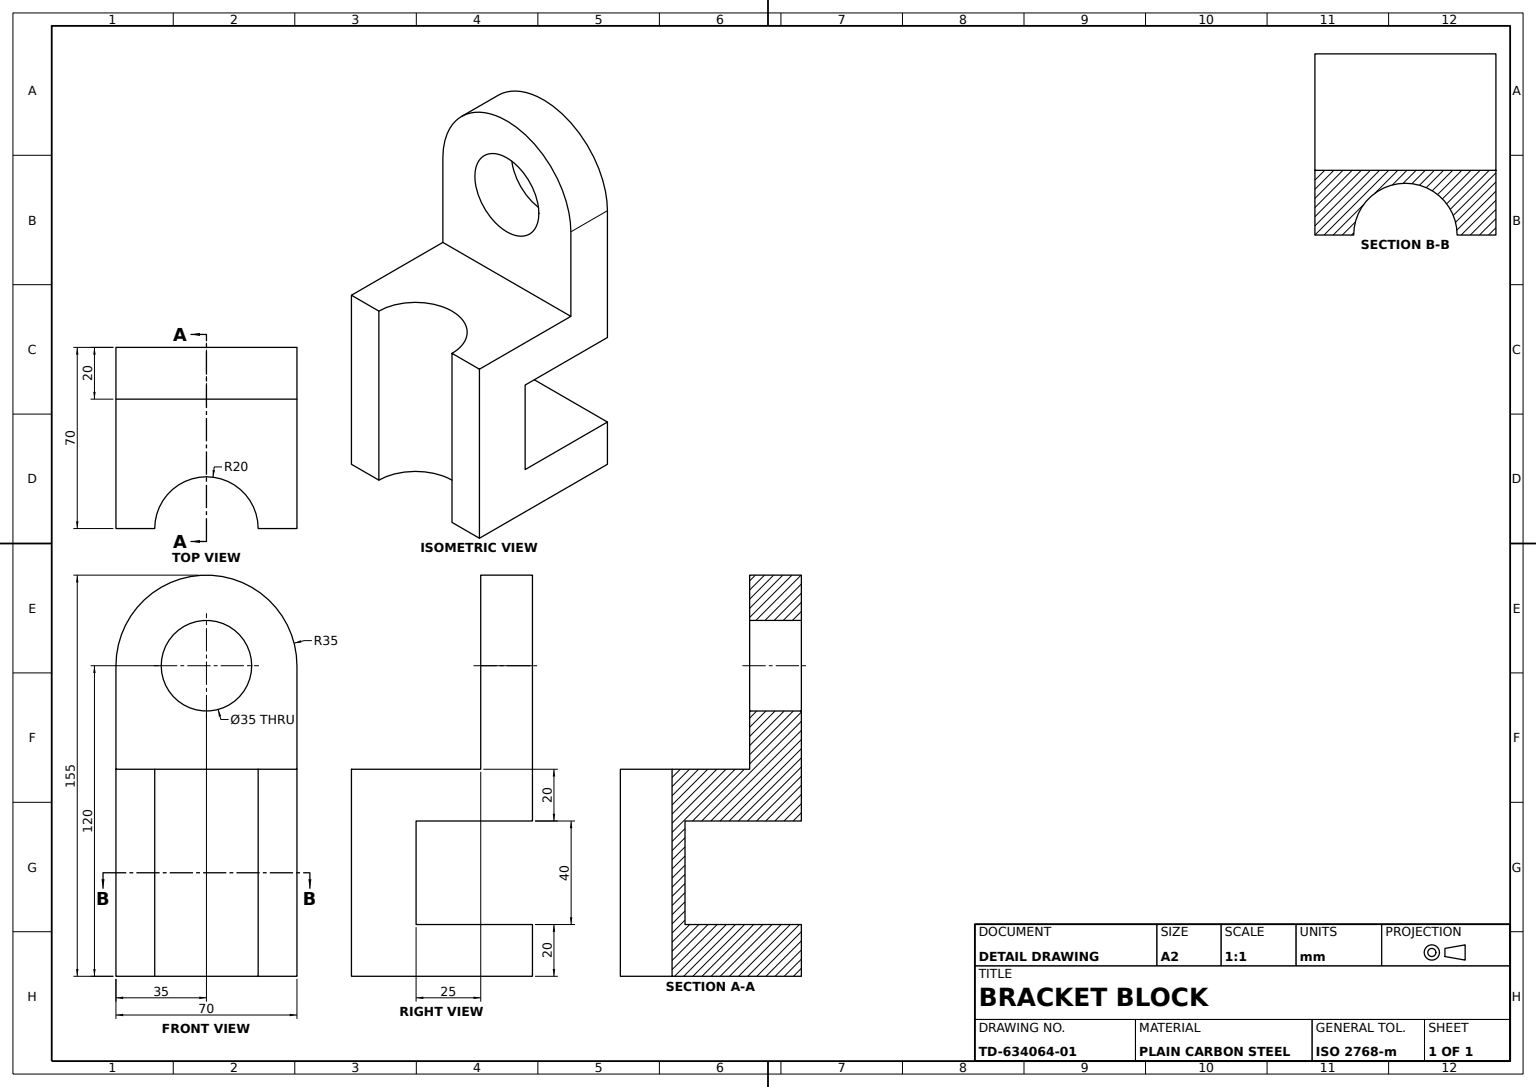
from build123d import *

# Parameters (mm, degrees)
LOWER_BODY_BLOCK_DEPTH = 20
UPRIGHT_START          = -60
UPRIGHT_WEB_DEPTH      = 60
UPPER_START            = -60
UPPER_BODY_BLOCK_DEPTH = 20
LIFTING_EYE_SKETCH_R   = 17.5
LIFTING_EYE_LUG_DEPTH  = 20


with BuildPart() as part:
    # Body Block Profile Sketch → Lower Body Block (new body)
    with BuildSketch(Plane(origin=(0, 0, 0), x_dir=(1, 0, 0), z_dir=(0, 1, 0))):
        with BuildLine():
            Line((20, -35), (35, -35))
            Line((35, -35), (35, 35))
            Line((35, 35), (-35, 35))
            Line((-35, 35), (-35, -35))
            Line((-35, -35), (-20, -35))
            ThreePointArc((-20, -35), (0, -15), (20, -35))
        make_face()
    extrude(amount=LOWER_BODY_BLOCK_DEPTH)

    # Upright Web Sketch → Upright Web (add)
    with BuildSketch(Plane(origin=(0, 20, 0), x_dir=(1, 0, 0), z_dir=(0, 1, 0)).offset(UPRIGHT_START)):
        with BuildLine():
            Line((-35, -35), (-20, -35))
            ThreePointArc((-20, -35), (0, -15), (20, -35))
            Line((20, -35), (35, -35))
            Line((35, -35), (35, -10))
            Line((35, -10), (-35, -10))
            Line((-35, -10), (-35, -35))
        make_face()
    extrude(amount=UPRIGHT_WEB_DEPTH)

    # Sketch2_2 → Upper Body Block (add)
    with BuildSketch(Plane(origin=(0, 0, 0), x_dir=(1, 0, 0), z_dir=(0, 1, 0)).offset(UPPER_START)):
        with BuildLine():
            Line((20, -35), (35, -35))
            Line((35, -35), (35, 35))
            Line((35, 35), (-35, 35))
            Line((-35, 35), (-35, -35))
            Line((-35, -35), (-20, -35))
            ThreePointArc((-20, -35), (0, -15), (20, -35))
        make_face()
    extrude(amount=UPPER_BODY_BLOCK_DEPTH)

    # Lifting Eye Sketch → Lifting Eye Lug (add)
    with BuildSketch(Plane(origin=(0, 0, -35), x_dir=(-1, 0, 0), z_dir=(0, 0, -1))):
        with BuildLine():
            Line((-35, 60), (-35, 20))
            Line((-35, 20), (35, 20))
            Line((35, 20), (35, 60))
            ThreePointArc((35, 60), (0, 95), (-35, 60))
        make_face()
        with Locations((0, 60)):
            Circle(LIFTING_EYE_SKETCH_R, mode=Mode.SUBTRACT)
    extrude(amount=-LIFTING_EYE_LUG_DEPTH)


solid = part.part
